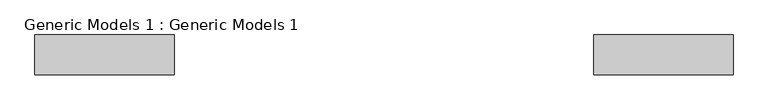
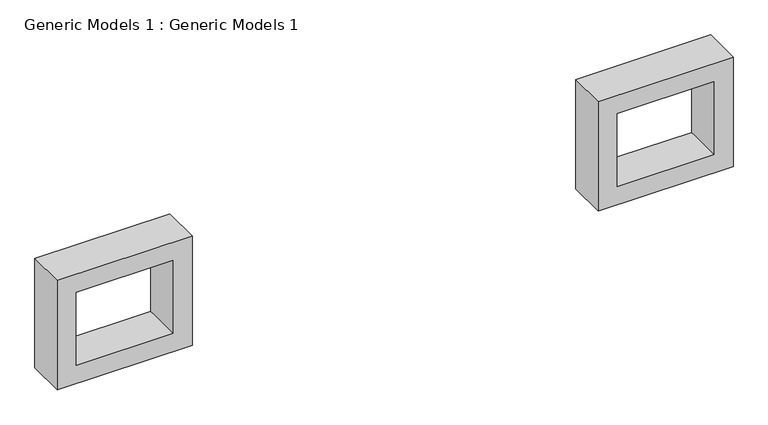
"""IFC4 building model written with IfcOpenShell, lengths in millimetres: proxy geometry, Generic Models 1 : Generic Models 1."""

from ifc_helpers import new_model, si_unit, frame, origin, place, context, project, spatial, polyline, outline, extrude, source, transform, mapped, element, save


def generic_models_1_generic_models_1_7471da39(model_context):
    return source(origin(), model_context, "Body", "SweptSolid", [
        extrude(outline(polyline([(5638.8, -3915.3833787), (5638.8, -6048.9833787), (3810.0, -6048.9833787), (3810.0, -3915.3833787), (5638.8, -3915.3833787)]), holes=[polyline([(5334.0, -4220.1833787), (4114.8, -4220.1833787), (4114.8, -5744.1833787), (5334.0, -5744.1833787), (5334.0, -4220.1833787)])]), frame((0.0, -10658.540066, 0.0), z_axis=(0.0, 1.0, 0.0), x_axis=(0.0, 0.0, 1.0)), (0.0, 0.0, 1.0), 609.6),
        extrude(outline(polyline([(5638.8, 4631.7166213), (5638.8, 2498.1166213), (3810.0, 2498.1166213), (3810.0, 4631.7166213), (5638.8, 4631.7166213)]), holes=[polyline([(5334.0, 4326.9166213), (4114.8, 4326.9166213), (4114.8, 2802.9166213), (5334.0, 2802.9166213), (5334.0, 4326.9166213)])]), frame((0.0, -10658.540066, 0.0), z_axis=(0.0, 1.0, 0.0), x_axis=(0.0, 0.0, 1.0)), (0.0, 0.0, 1.0), 609.6),
    ])


if __name__ == "__main__":
    model = new_model("IFC4")
    model_context = context("Model", 3, world=origin())
    ifc_project = project(units=[si_unit("LENGTHUNIT", "METRE", prefix="MILLI")], contexts=[model_context])
    site = spatial("IfcSite", under=ifc_project)
    building = spatial("IfcBuilding", under=site)
    placement = place(None, origin())
    generic_models_1_generic_models_1_shape = generic_models_1_generic_models_1_7471da39(model_context)
    element("IfcBuildingElementProxy", 1, Name="Generic Models 1 : Generic Models 1", ObjectType="Generic Models 1 : Generic Models 1", at=placement, inside=building, context=model_context, shape_type="MappedRepresentation", body=[
        mapped(generic_models_1_generic_models_1_shape, transform((0.0, 0.0, 0.0), x_axis=(1.0, 0.0, 0.0), y_axis=(0.0, 1.0, 0.0), z_axis=(0.0, 0.0, 1.0))),
    ])
    save(model, "model.ifc")

# Revit data of these elements
# Element 1 (IfcBuildingElementProxy, "Generic Models 1 : Generic Models 1")
#   Materials on its faces: "grey"
# Materials
#   "grey": class "Generic", colour RGB 33 34 34, transparency 0, Cost = 0
